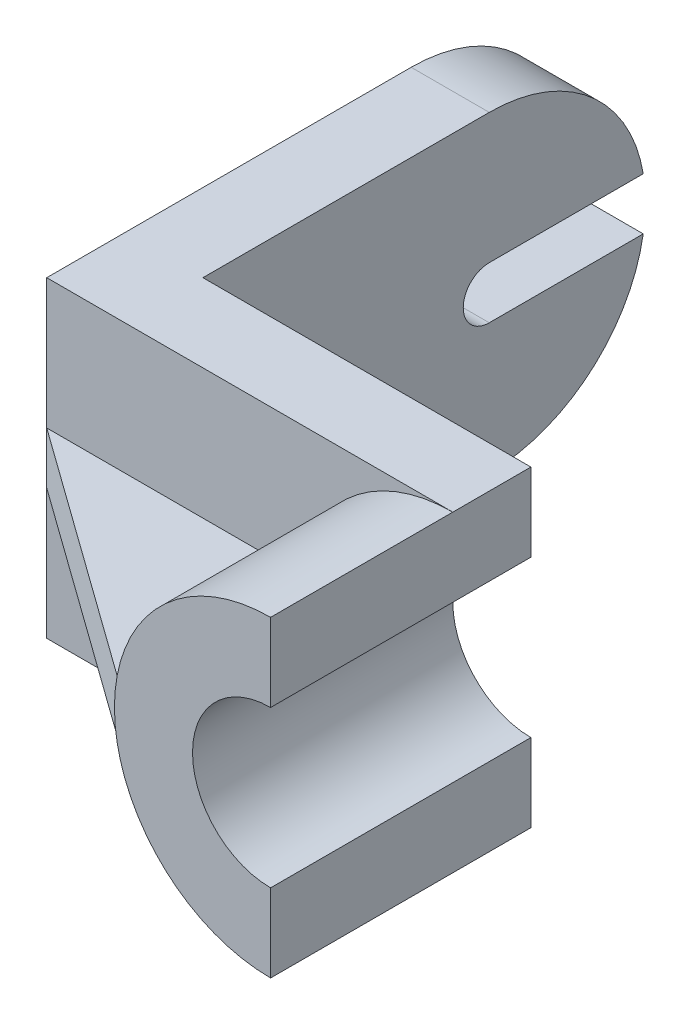
ISO-10303-21;
HEADER;
FILE_DESCRIPTION(('STEP AP214'),'2;1');
FILE_NAME('part.step','',(''),(''),'','','');
FILE_SCHEMA(('AUTOMOTIVE_DESIGN { 1 0 10303 214 1 1 1 1 }'));
ENDSEC;
DATA;
#1=APPLICATION_CONTEXT('core data for automotive mechanical design processes');
#2=APPLICATION_PROTOCOL_DEFINITION('international standard','automotive_design',2000,#1);
#3=PRODUCT_CONTEXT('',#1,'mechanical');
#4=PRODUCT('Part','Part','',(#3));
#5=PRODUCT_RELATED_PRODUCT_CATEGORY('part','',(#4));
#6=PRODUCT_DEFINITION_FORMATION('','',#4);
#7=PRODUCT_DEFINITION_CONTEXT('part definition',#1,'design');
#8=PRODUCT_DEFINITION('design','',#6,#7);
#9=PRODUCT_DEFINITION_SHAPE('','',#8);
#10=(LENGTH_UNIT() NAMED_UNIT(*) SI_UNIT(.MILLI.,.METRE.));
#11=(NAMED_UNIT(*) PLANE_ANGLE_UNIT() SI_UNIT($,.RADIAN.));
#12=(NAMED_UNIT(*) SI_UNIT($,.STERADIAN.) SOLID_ANGLE_UNIT());
#13=UNCERTAINTY_MEASURE_WITH_UNIT(LENGTH_MEASURE(1.E-05),#10,'distance_accuracy_value','');
#14=(GEOMETRIC_REPRESENTATION_CONTEXT(3) GLOBAL_UNCERTAINTY_ASSIGNED_CONTEXT((#13)) GLOBAL_UNIT_ASSIGNED_CONTEXT((#10,
#11,#12)) REPRESENTATION_CONTEXT('',''));
#15=CARTESIAN_POINT('',(0.,0.,0.));
#16=DIRECTION('',(0.,0.,1.));
#17=DIRECTION('',(1.,0.,0.));
#18=AXIS2_PLACEMENT_3D('',#15,#16,#17);
#19=CARTESIAN_POINT('',(15.,-60.,0.));
#20=DIRECTION('',(0.,0.,-1.));
#21=DIRECTION('',(-1.,0.,0.));
#22=AXIS2_PLACEMENT_3D('',#19,#20,#21);
#23=PLANE('',#22);
#24=DIRECTION('',(-1.,0.,0.));
#25=VECTOR('',#24,1.);
#26=CARTESIAN_POINT('',(15.,-25.,0.));
#27=LINE('',#26,#25);
#28=CARTESIAN_POINT('',(48.4196010845019,-25.,0.));
#29=VERTEX_POINT('',#28);
#30=CARTESIAN_POINT('',(0.,-25.,0.));
#31=VERTEX_POINT('',#30);
#32=EDGE_CURVE('E148',#29,#31,#27,.T.);
#33=ORIENTED_EDGE('',*,*,#32,.F.);
#34=CARTESIAN_POINT('',(78.,-30.,0.));
#35=DIRECTION('',(0.,0.,1.));
#36=DIRECTION('',(1.,0.,0.));
#37=AXIS2_PLACEMENT_3D('',#34,#35,#36);
#38=CIRCLE('',#37,30.);
#39=CARTESIAN_POINT('',(78.,0.,0.));
#40=VERTEX_POINT('',#39);
#41=EDGE_CURVE('E246',#40,#29,#38,.T.);
#42=ORIENTED_EDGE('',*,*,#41,.F.);
#43=DIRECTION('',(-1.,0.,0.));
#44=VECTOR('',#43,1.);
#45=CARTESIAN_POINT('',(15.,0.,0.));
#46=LINE('',#45,#44);
#47=CARTESIAN_POINT('',(0.,0.,0.));
#48=VERTEX_POINT('',#47);
#49=EDGE_CURVE('E179',#40,#48,#46,.T.);
#50=ORIENTED_EDGE('',*,*,#49,.T.);
#51=DIRECTION('',(0.,-1.,0.));
#52=VECTOR('',#51,1.);
#53=CARTESIAN_POINT('',(0.,-60.,0.));
#54=LINE('',#53,#52);
#55=EDGE_CURVE('E173',#48,#31,#54,.T.);
#56=ORIENTED_EDGE('',*,*,#55,.T.);
#57=EDGE_LOOP('',(#33,#42,#50,#56));
#58=FACE_BOUND('',#57,.T.);
#59=ADVANCED_FACE('F39',(#58),#23,.F.);
#60=CARTESIAN_POINT('',(15.,-30.,-70.));
#61=DIRECTION('',(-1.,0.,0.));
#62=DIRECTION('',(0.,0.,1.));
#63=AXIS2_PLACEMENT_3D('',#60,#61,#62);
#64=CYLINDRICAL_SURFACE('',#63,30.);
#65=DIRECTION('',(1.,0.,0.));
#66=VECTOR('',#65,1.);
#67=CARTESIAN_POINT('',(0.,-25.,-99.5803989154981));
#68=LINE('',#67,#66);
#69=CARTESIAN_POINT('',(0.,-25.,-99.5803989154981));
#70=VERTEX_POINT('',#69);
#71=CARTESIAN_POINT('',(15.,-25.,-99.5803989154981));
#72=VERTEX_POINT('',#71);
#73=EDGE_CURVE('E219',#70,#72,#68,.T.);
#74=ORIENTED_EDGE('',*,*,#73,.F.);
#75=CARTESIAN_POINT('',(0.,-30.,-70.));
#76=DIRECTION('',(-1.,0.,0.));
#77=DIRECTION('',(0.,0.,1.));
#78=AXIS2_PLACEMENT_3D('',#75,#76,#77);
#79=CIRCLE('',#78,30.);
#80=CARTESIAN_POINT('',(0.,0.,-70.));
#81=VERTEX_POINT('',#80);
#82=EDGE_CURVE('E216',#81,#70,#79,.T.);
#83=ORIENTED_EDGE('',*,*,#82,.F.);
#84=DIRECTION('',(-1.,0.,0.));
#85=VECTOR('',#84,1.);
#86=CARTESIAN_POINT('',(15.,0.,-70.));
#87=LINE('',#86,#85);
#88=CARTESIAN_POINT('',(15.,0.,-70.));
#89=VERTEX_POINT('',#88);
#90=EDGE_CURVE('E194',#89,#81,#87,.T.);
#91=ORIENTED_EDGE('',*,*,#90,.F.);
#92=CARTESIAN_POINT('',(15.,-30.,-70.));
#93=DIRECTION('',(-1.,0.,0.));
#94=DIRECTION('',(0.,0.,1.));
#95=AXIS2_PLACEMENT_3D('',#92,#93,#94);
#96=CIRCLE('',#95,30.);
#97=EDGE_CURVE('E184',#89,#72,#96,.T.);
#98=ORIENTED_EDGE('',*,*,#97,.T.);
#99=EDGE_LOOP('',(#74,#83,#91,#98));
#100=FACE_BOUND('',#99,.T.);
#101=ADVANCED_FACE('F273',(#100),#64,.T.);
#102=CARTESIAN_POINT('',(48.4196010845019,-35.,0.));
#103=VERTEX_POINT('',#102);
#104=CARTESIAN_POINT('',(77.9999999999997,-60.,0.));
#105=VERTEX_POINT('',#104);
#106=EDGE_CURVE('E305',#103,#105,#38,.T.);
#107=ORIENTED_EDGE('',*,*,#106,.F.);
#108=DIRECTION('',(-1.,0.,0.));
#109=VECTOR('',#108,1.);
#110=CARTESIAN_POINT('',(15.,-35.,0.));
#111=LINE('',#110,#109);
#112=CARTESIAN_POINT('',(0.,-35.,0.));
#113=VERTEX_POINT('',#112);
#114=EDGE_CURVE('E303',#103,#113,#111,.T.);
#115=ORIENTED_EDGE('',*,*,#114,.T.);
#116=CARTESIAN_POINT('',(0.,-60.,0.));
#117=VERTEX_POINT('',#116);
#118=EDGE_CURVE('E174',#113,#117,#54,.T.);
#119=ORIENTED_EDGE('',*,*,#118,.T.);
#120=DIRECTION('',(-1.,0.,0.));
#121=VECTOR('',#120,1.);
#122=CARTESIAN_POINT('',(15.,-60.,0.));
#123=LINE('',#122,#121);
#124=EDGE_CURVE('E11',#105,#117,#123,.T.);
#125=ORIENTED_EDGE('',*,*,#124,.F.);
#126=EDGE_LOOP('',(#107,#115,#119,#125));
#127=FACE_BOUND('',#126,.T.);
#128=ADVANCED_FACE('F41',(#127),#23,.F.);
#129=CARTESIAN_POINT('',(15.,-60.,-70.));
#130=DIRECTION('',(0.,1.,0.));
#131=DIRECTION('',(0.,0.,1.));
#132=AXIS2_PLACEMENT_3D('',#129,#130,#131);
#133=PLANE('',#132);
#134=DIRECTION('',(0.,0.,-1.));
#135=VECTOR('',#134,1.);
#136=CARTESIAN_POINT('',(15.,-60.,-70.));
#137=LINE('',#136,#135);
#138=CARTESIAN_POINT('',(15.,-60.,-15.));
#139=VERTEX_POINT('',#138);
#140=CARTESIAN_POINT('',(15.,-60.,-70.));
#141=VERTEX_POINT('',#140);
#142=EDGE_CURVE('E192',#139,#141,#137,.T.);
#143=ORIENTED_EDGE('',*,*,#142,.F.);
#144=DIRECTION('',(1.,0.,0.));
#145=VECTOR('',#144,1.);
#146=CARTESIAN_POINT('',(78.,-60.,-15.));
#147=LINE('',#146,#145);
#148=CARTESIAN_POINT('',(78.,-60.,-15.));
#149=VERTEX_POINT('',#148);
#150=EDGE_CURVE('E240',#139,#149,#147,.T.);
#151=ORIENTED_EDGE('',*,*,#150,.T.);
#152=DIRECTION('',(0.,0.,1.));
#153=VECTOR('',#152,1.);
#154=CARTESIAN_POINT('',(78.,-60.,-15.));
#155=LINE('',#154,#153);
#156=EDGE_CURVE('E243',#149,#105,#155,.T.);
#157=ORIENTED_EDGE('',*,*,#156,.T.);
#158=ORIENTED_EDGE('',*,*,#124,.T.);
#159=DIRECTION('',(0.,0.,-1.));
#160=VECTOR('',#159,1.);
#161=CARTESIAN_POINT('',(0.,-60.,-70.));
#162=LINE('',#161,#160);
#163=CARTESIAN_POINT('',(0.,-60.,-70.));
#164=VERTEX_POINT('',#163);
#165=EDGE_CURVE('E181',#117,#164,#162,.T.);
#166=ORIENTED_EDGE('',*,*,#165,.T.);
#167=DIRECTION('',(-1.,0.,0.));
#168=VECTOR('',#167,1.);
#169=CARTESIAN_POINT('',(15.,-60.,-70.));
#170=LINE('',#169,#168);
#171=EDGE_CURVE('E50',#141,#164,#170,.T.);
#172=ORIENTED_EDGE('',*,*,#171,.F.);
#173=EDGE_LOOP('',(#143,#151,#157,#158,#166,#172));
#174=FACE_BOUND('',#173,.T.);
#175=ADVANCED_FACE('F210',(#174),#133,.F.);
#176=CARTESIAN_POINT('',(15.,0.,0.));
#177=DIRECTION('',(0.,-1.,0.));
#178=DIRECTION('',(0.,0.,-1.));
#179=AXIS2_PLACEMENT_3D('',#176,#177,#178);
#180=PLANE('',#179);
#181=DIRECTION('',(0.,0.,1.));
#182=VECTOR('',#181,1.);
#183=CARTESIAN_POINT('',(0.,0.,0.));
#184=LINE('',#183,#182);
#185=EDGE_CURVE('E182',#81,#48,#184,.T.);
#186=ORIENTED_EDGE('',*,*,#185,.T.);
#187=ORIENTED_EDGE('',*,*,#49,.F.);
#188=DIRECTION('',(0.,0.,1.));
#189=VECTOR('',#188,1.);
#190=CARTESIAN_POINT('',(78.,0.,-15.));
#191=LINE('',#190,#189);
#192=CARTESIAN_POINT('',(78.,0.,-15.));
#193=VERTEX_POINT('',#192);
#194=EDGE_CURVE('E237',#193,#40,#191,.T.);
#195=ORIENTED_EDGE('',*,*,#194,.F.);
#196=DIRECTION('',(-1.,0.,0.));
#197=VECTOR('',#196,1.);
#198=CARTESIAN_POINT('',(0.,0.,-15.));
#199=LINE('',#198,#197);
#200=CARTESIAN_POINT('',(15.,0.,-15.));
#201=VERTEX_POINT('',#200);
#202=EDGE_CURVE('E236',#193,#201,#199,.T.);
#203=ORIENTED_EDGE('',*,*,#202,.T.);
#204=DIRECTION('',(0.,0.,1.));
#205=VECTOR('',#204,1.);
#206=CARTESIAN_POINT('',(15.,0.,0.));
#207=LINE('',#206,#205);
#208=EDGE_CURVE('E190',#89,#201,#207,.T.);
#209=ORIENTED_EDGE('',*,*,#208,.F.);
#210=ORIENTED_EDGE('',*,*,#90,.T.);
#211=EDGE_LOOP('',(#186,#187,#195,#203,#209,#210));
#212=FACE_BOUND('',#211,.T.);
#213=ADVANCED_FACE('F245',(#212),#180,.F.);
#214=CARTESIAN_POINT('',(15.,0.,0.));
#215=DIRECTION('',(-1.,0.,0.));
#216=DIRECTION('',(0.,0.,1.));
#217=AXIS2_PLACEMENT_3D('',#214,#215,#216);
#218=PLANE('',#217);
#219=DIRECTION('',(0.,0.,-1.));
#220=VECTOR('',#219,1.);
#221=CARTESIAN_POINT('',(15.,-35.,-70.));
#222=LINE('',#221,#220);
#223=CARTESIAN_POINT('',(15.,-35.,-70.));
#224=VERTEX_POINT('',#223);
#225=CARTESIAN_POINT('',(15.,-35.,-99.5803989154981));
#226=VERTEX_POINT('',#225);
#227=EDGE_CURVE('E261',#224,#226,#222,.T.);
#228=ORIENTED_EDGE('',*,*,#227,.F.);
#229=CARTESIAN_POINT('',(15.,-30.,-70.));
#230=DIRECTION('',(1.,0.,0.));
#231=DIRECTION('',(0.,0.,-1.));
#232=AXIS2_PLACEMENT_3D('',#229,#230,#231);
#233=CIRCLE('',#232,5.);
#234=CARTESIAN_POINT('',(15.,-25.,-70.));
#235=VERTEX_POINT('',#234);
#236=EDGE_CURVE('E238',#235,#224,#233,.T.);
#237=ORIENTED_EDGE('',*,*,#236,.F.);
#238=DIRECTION('',(0.,0.,1.));
#239=VECTOR('',#238,1.);
#240=CARTESIAN_POINT('',(15.,-25.,-70.));
#241=LINE('',#240,#239);
#242=EDGE_CURVE('E254',#72,#235,#241,.T.);
#243=ORIENTED_EDGE('',*,*,#242,.F.);
#244=ORIENTED_EDGE('',*,*,#97,.F.);
#245=ORIENTED_EDGE('',*,*,#208,.T.);
#246=DIRECTION('',(0.,-1.,0.));
#247=VECTOR('',#246,1.);
#248=CARTESIAN_POINT('',(15.,0.,-15.));
#249=LINE('',#248,#247);
#250=EDGE_CURVE('E65',#201,#139,#249,.T.);
#251=ORIENTED_EDGE('',*,*,#250,.T.);
#252=ORIENTED_EDGE('',*,*,#142,.T.);
#253=EDGE_CURVE('E203',#226,#141,#96,.T.);
#254=ORIENTED_EDGE('',*,*,#253,.F.);
#255=EDGE_LOOP('',(#228,#237,#243,#244,#245,#251,#252,#254));
#256=FACE_BOUND('',#255,.T.);
#257=ADVANCED_FACE('F228',(#256),#218,.F.);
#258=CARTESIAN_POINT('',(0.,0.,0.));
#259=DIRECTION('',(-1.,0.,0.));
#260=DIRECTION('',(0.,0.,1.));
#261=AXIS2_PLACEMENT_3D('',#258,#259,#260);
#262=PLANE('',#261);
#263=ORIENTED_EDGE('',*,*,#118,.F.);
#264=DIRECTION('',(0.,-1.,0.));
#265=VECTOR('',#264,1.);
#266=CARTESIAN_POINT('',(0.,0.,0.));
#267=LINE('',#266,#265);
#268=EDGE_CURVE('E165',#113,#31,#267,.F.);
#269=ORIENTED_EDGE('',*,*,#268,.T.);
#270=ORIENTED_EDGE('',*,*,#55,.F.);
#271=ORIENTED_EDGE('',*,*,#185,.F.);
#272=ORIENTED_EDGE('',*,*,#82,.T.);
#273=DIRECTION('',(0.,0.,1.));
#274=VECTOR('',#273,1.);
#275=CARTESIAN_POINT('',(0.,-25.,-70.));
#276=LINE('',#275,#274);
#277=CARTESIAN_POINT('',(0.,-25.,-70.));
#278=VERTEX_POINT('',#277);
#279=EDGE_CURVE('E253',#70,#278,#276,.T.);
#280=ORIENTED_EDGE('',*,*,#279,.T.);
#281=CARTESIAN_POINT('',(0.,-30.,-70.));
#282=DIRECTION('',(1.,0.,0.));
#283=DIRECTION('',(0.,0.,-1.));
#284=AXIS2_PLACEMENT_3D('',#281,#282,#283);
#285=CIRCLE('',#284,5.);
#286=CARTESIAN_POINT('',(0.,-35.,-70.));
#287=VERTEX_POINT('',#286);
#288=EDGE_CURVE('E252',#278,#287,#285,.T.);
#289=ORIENTED_EDGE('',*,*,#288,.T.);
#290=DIRECTION('',(0.,0.,-1.));
#291=VECTOR('',#290,1.);
#292=CARTESIAN_POINT('',(0.,-35.,-70.));
#293=LINE('',#292,#291);
#294=CARTESIAN_POINT('',(0.,-35.,-99.5803989154981));
#295=VERTEX_POINT('',#294);
#296=EDGE_CURVE('E213',#287,#295,#293,.T.);
#297=ORIENTED_EDGE('',*,*,#296,.T.);
#298=EDGE_CURVE('E205',#295,#164,#79,.T.);
#299=ORIENTED_EDGE('',*,*,#298,.T.);
#300=ORIENTED_EDGE('',*,*,#165,.F.);
#301=EDGE_LOOP('',(#263,#269,#270,#271,#272,#280,#289,#297,#299,#300));
#302=FACE_BOUND('',#301,.T.);
#303=ADVANCED_FACE('F175',(#302),#262,.T.);
#304=DIRECTION('',(1.,0.,0.));
#305=VECTOR('',#304,1.);
#306=CARTESIAN_POINT('',(0.,-35.,-99.5803989154981));
#307=LINE('',#306,#305);
#308=EDGE_CURVE('E267',#295,#226,#307,.T.);
#309=ORIENTED_EDGE('',*,*,#308,.T.);
#310=ORIENTED_EDGE('',*,*,#253,.T.);
#311=ORIENTED_EDGE('',*,*,#171,.T.);
#312=ORIENTED_EDGE('',*,*,#298,.F.);
#313=EDGE_LOOP('',(#309,#310,#311,#312));
#314=FACE_BOUND('',#313,.T.);
#315=ADVANCED_FACE('F202',(#314),#64,.T.);
#316=CARTESIAN_POINT('',(0.,-30.,-70.));
#317=DIRECTION('',(1.,0.,0.));
#318=DIRECTION('',(0.,0.,-1.));
#319=AXIS2_PLACEMENT_3D('',#316,#317,#318);
#320=CYLINDRICAL_SURFACE('',#319,5.);
#321=ORIENTED_EDGE('',*,*,#236,.T.);
#322=DIRECTION('',(1.,0.,0.));
#323=VECTOR('',#322,1.);
#324=CARTESIAN_POINT('',(0.,-35.,-70.));
#325=LINE('',#324,#323);
#326=EDGE_CURVE('E259',#287,#224,#325,.T.);
#327=ORIENTED_EDGE('',*,*,#326,.F.);
#328=ORIENTED_EDGE('',*,*,#288,.F.);
#329=DIRECTION('',(1.,0.,0.));
#330=VECTOR('',#329,1.);
#331=CARTESIAN_POINT('',(0.,-25.,-70.));
#332=LINE('',#331,#330);
#333=EDGE_CURVE('E220',#278,#235,#332,.T.);
#334=ORIENTED_EDGE('',*,*,#333,.T.);
#335=EDGE_LOOP('',(#321,#327,#328,#334));
#336=FACE_BOUND('',#335,.T.);
#337=ADVANCED_FACE('F275',(#336),#320,.F.);
#338=CARTESIAN_POINT('',(0.,-25.,-70.));
#339=DIRECTION('',(0.,1.,0.));
#340=DIRECTION('',(0.,0.,1.));
#341=AXIS2_PLACEMENT_3D('',#338,#339,#340);
#342=PLANE('',#341);
#343=ORIENTED_EDGE('',*,*,#242,.T.);
#344=ORIENTED_EDGE('',*,*,#333,.F.);
#345=ORIENTED_EDGE('',*,*,#279,.F.);
#346=ORIENTED_EDGE('',*,*,#73,.T.);
#347=EDGE_LOOP('',(#343,#344,#345,#346));
#348=FACE_BOUND('',#347,.T.);
#349=ADVANCED_FACE('F279',(#348),#342,.F.);
#350=CARTESIAN_POINT('',(0.,-35.,-70.));
#351=DIRECTION('',(0.,-1.,0.));
#352=DIRECTION('',(0.,0.,-1.));
#353=AXIS2_PLACEMENT_3D('',#350,#351,#352);
#354=PLANE('',#353);
#355=ORIENTED_EDGE('',*,*,#227,.T.);
#356=ORIENTED_EDGE('',*,*,#308,.F.);
#357=ORIENTED_EDGE('',*,*,#296,.F.);
#358=ORIENTED_EDGE('',*,*,#326,.T.);
#359=EDGE_LOOP('',(#355,#356,#357,#358));
#360=FACE_BOUND('',#359,.T.);
#361=ADVANCED_FACE('F270',(#360),#354,.F.);
#362=CARTESIAN_POINT('',(0.,0.,-15.));
#363=DIRECTION('',(0.,0.,-1.));
#364=DIRECTION('',(-1.,0.,0.));
#365=AXIS2_PLACEMENT_3D('',#362,#363,#364);
#366=PLANE('',#365);
#367=ORIENTED_EDGE('',*,*,#150,.F.);
#368=ORIENTED_EDGE('',*,*,#250,.F.);
#369=ORIENTED_EDGE('',*,*,#202,.F.);
#370=DIRECTION('',(0.,-1.,0.));
#371=VECTOR('',#370,1.);
#372=CARTESIAN_POINT('',(78.,-15.,-15.));
#373=LINE('',#372,#371);
#374=CARTESIAN_POINT('',(78.,-15.,-15.));
#375=VERTEX_POINT('',#374);
#376=EDGE_CURVE('E176',#193,#375,#373,.T.);
#377=ORIENTED_EDGE('',*,*,#376,.T.);
#378=CARTESIAN_POINT('',(77.9999999999997,-30.,-15.));
#379=DIRECTION('',(0.,0.,1.));
#380=DIRECTION('',(-1.,0.,0.));
#381=AXIS2_PLACEMENT_3D('',#378,#379,#380);
#382=CIRCLE('',#381,15.);
#383=CARTESIAN_POINT('',(77.9999999999997,-45.,-15.));
#384=VERTEX_POINT('',#383);
#385=EDGE_CURVE('E325',#375,#384,#382,.T.);
#386=ORIENTED_EDGE('',*,*,#385,.T.);
#387=DIRECTION('',(0.,-1.,0.));
#388=VECTOR('',#387,1.);
#389=CARTESIAN_POINT('',(77.9999999999997,-60.,-15.));
#390=LINE('',#389,#388);
#391=EDGE_CURVE('E316',#384,#149,#390,.T.);
#392=ORIENTED_EDGE('',*,*,#391,.T.);
#393=EDGE_LOOP('',(#367,#368,#369,#377,#386,#392));
#394=FACE_BOUND('',#393,.T.);
#395=ADVANCED_FACE('F234',(#394),#366,.T.);
#396=CARTESIAN_POINT('',(77.9999999999998,-30.,35.));
#397=DIRECTION('',(0.,0.,-1.));
#398=DIRECTION('',(-1.,0.,0.));
#399=AXIS2_PLACEMENT_3D('',#396,#397,#398);
#400=CYLINDRICAL_SURFACE('',#399,30.);
#401=DIRECTION('',(0.,0.,-1.));
#402=VECTOR('',#401,1.);
#403=CARTESIAN_POINT('',(48.4196010845018,-35.,35.));
#404=LINE('',#403,#402);
#405=CARTESIAN_POINT('',(48.4196010845018,-35.,34.7742237705084));
#406=VERTEX_POINT('',#405);
#407=EDGE_CURVE('E333',#103,#406,#404,.F.);
#408=ORIENTED_EDGE('',*,*,#407,.F.);
#409=ORIENTED_EDGE('',*,*,#106,.T.);
#410=DIRECTION('',(0.,0.,-1.));
#411=VECTOR('',#410,1.);
#412=CARTESIAN_POINT('',(77.9999999999997,-60.,35.));
#413=LINE('',#412,#411);
#414=CARTESIAN_POINT('',(77.9999999999997,-60.,35.));
#415=VERTEX_POINT('',#414);
#416=EDGE_CURVE('E310',#415,#105,#413,.T.);
#417=ORIENTED_EDGE('',*,*,#416,.F.);
#418=CARTESIAN_POINT('',(77.9999999999998,-30.,35.));
#419=DIRECTION('',(0.,0.,-1.));
#420=DIRECTION('',(-1.,0.,0.));
#421=AXIS2_PLACEMENT_3D('',#418,#419,#420);
#422=CIRCLE('',#421,30.);
#423=CARTESIAN_POINT('',(78.,0.,35.));
#424=VERTEX_POINT('',#423);
#425=EDGE_CURVE('E322',#415,#424,#422,.T.);
#426=ORIENTED_EDGE('',*,*,#425,.T.);
#427=DIRECTION('',(0.,0.,-1.));
#428=VECTOR('',#427,1.);
#429=CARTESIAN_POINT('',(78.,0.,35.));
#430=LINE('',#429,#428);
#431=EDGE_CURVE('E311',#424,#40,#430,.T.);
#432=ORIENTED_EDGE('',*,*,#431,.T.);
#433=ORIENTED_EDGE('',*,*,#41,.T.);
#434=DIRECTION('',(0.,0.,-1.));
#435=VECTOR('',#434,1.);
#436=CARTESIAN_POINT('',(48.4196010845018,-25.,35.));
#437=LINE('',#436,#435);
#438=CARTESIAN_POINT('',(48.4196010845018,-25.,34.7742237705084));
#439=VERTEX_POINT('',#438);
#440=EDGE_CURVE('E153',#29,#439,#437,.F.);
#441=ORIENTED_EDGE('',*,*,#440,.T.);
#442=CARTESIAN_POINT('',(77.9999999999998,-30.,56.0184180238493));
#443=DIRECTION('',(0.583333333333333,0.,-0.812232862067414));
#444=DIRECTION('',(-0.812232862067414,0.,-0.583333333333333));
#445=AXIS2_PLACEMENT_3D('',#442,#443,#444);
#446=ELLIPSE('',#445,36.9352206750656,30.);
#447=EDGE_CURVE('E170',#406,#439,#446,.T.);
#448=ORIENTED_EDGE('',*,*,#447,.F.);
#449=EDGE_LOOP('',(#408,#409,#417,#426,#432,#433,#441,#448));
#450=FACE_BOUND('',#449,.T.);
#451=ADVANCED_FACE('F338',(#450),#400,.T.);
#452=CARTESIAN_POINT('',(77.9999999999997,-60.,35.));
#453=DIRECTION('',(1.,0.,0.));
#454=DIRECTION('',(0.,0.,-1.));
#455=AXIS2_PLACEMENT_3D('',#452,#453,#454);
#456=PLANE('',#455);
#457=ORIENTED_EDGE('',*,*,#391,.F.);
#458=DIRECTION('',(0.,0.,-1.));
#459=VECTOR('',#458,1.);
#460=CARTESIAN_POINT('',(77.9999999999997,-45.,35.));
#461=LINE('',#460,#459);
#462=CARTESIAN_POINT('',(77.9999999999997,-45.,35.));
#463=VERTEX_POINT('',#462);
#464=EDGE_CURVE('E308',#463,#384,#461,.T.);
#465=ORIENTED_EDGE('',*,*,#464,.F.);
#466=DIRECTION('',(0.,-1.,0.));
#467=VECTOR('',#466,1.);
#468=CARTESIAN_POINT('',(77.9999999999997,-60.,35.));
#469=LINE('',#468,#467);
#470=EDGE_CURVE('E314',#463,#415,#469,.T.);
#471=ORIENTED_EDGE('',*,*,#470,.T.);
#472=ORIENTED_EDGE('',*,*,#416,.T.);
#473=ORIENTED_EDGE('',*,*,#156,.F.);
#474=EDGE_LOOP('',(#457,#465,#471,#472,#473));
#475=FACE_BOUND('',#474,.T.);
#476=ADVANCED_FACE('F353',(#475),#456,.T.);
#477=CARTESIAN_POINT('',(77.9999999999997,-30.,35.));
#478=DIRECTION('',(0.,0.,-1.));
#479=DIRECTION('',(-1.,0.,0.));
#480=AXIS2_PLACEMENT_3D('',#477,#478,#479);
#481=CYLINDRICAL_SURFACE('',#480,15.);
#482=ORIENTED_EDGE('',*,*,#464,.T.);
#483=ORIENTED_EDGE('',*,*,#385,.F.);
#484=DIRECTION('',(0.,0.,-1.));
#485=VECTOR('',#484,1.);
#486=CARTESIAN_POINT('',(78.,-15.,35.));
#487=LINE('',#486,#485);
#488=CARTESIAN_POINT('',(78.,-15.,35.));
#489=VERTEX_POINT('',#488);
#490=EDGE_CURVE('E313',#489,#375,#487,.T.);
#491=ORIENTED_EDGE('',*,*,#490,.F.);
#492=CARTESIAN_POINT('',(77.9999999999997,-30.,35.));
#493=DIRECTION('',(0.,0.,1.));
#494=DIRECTION('',(-1.,0.,0.));
#495=AXIS2_PLACEMENT_3D('',#492,#493,#494);
#496=CIRCLE('',#495,15.);
#497=EDGE_CURVE('E330',#489,#463,#496,.T.);
#498=ORIENTED_EDGE('',*,*,#497,.T.);
#499=EDGE_LOOP('',(#482,#483,#491,#498));
#500=FACE_BOUND('',#499,.T.);
#501=ADVANCED_FACE('F352',(#500),#481,.F.);
#502=CARTESIAN_POINT('',(78.,-15.,35.));
#503=DIRECTION('',(1.,0.,0.));
#504=DIRECTION('',(0.,1.,0.));
#505=AXIS2_PLACEMENT_3D('',#502,#503,#504);
#506=PLANE('',#505);
#507=ORIENTED_EDGE('',*,*,#376,.F.);
#508=ORIENTED_EDGE('',*,*,#194,.T.);
#509=ORIENTED_EDGE('',*,*,#431,.F.);
#510=DIRECTION('',(0.,-1.,0.));
#511=VECTOR('',#510,1.);
#512=CARTESIAN_POINT('',(78.,-15.,35.));
#513=LINE('',#512,#511);
#514=EDGE_CURVE('E327',#424,#489,#513,.T.);
#515=ORIENTED_EDGE('',*,*,#514,.T.);
#516=ORIENTED_EDGE('',*,*,#490,.T.);
#517=EDGE_LOOP('',(#507,#508,#509,#515,#516));
#518=FACE_BOUND('',#517,.T.);
#519=ADVANCED_FACE('F341',(#518),#506,.T.);
#520=CARTESIAN_POINT('',(77.9999999999998,-30.,35.));
#521=DIRECTION('',(0.,0.,-1.));
#522=DIRECTION('',(-1.,0.,0.));
#523=AXIS2_PLACEMENT_3D('',#520,#521,#522);
#524=PLANE('',#523);
#525=ORIENTED_EDGE('',*,*,#470,.F.);
#526=ORIENTED_EDGE('',*,*,#497,.F.);
#527=ORIENTED_EDGE('',*,*,#514,.F.);
#528=ORIENTED_EDGE('',*,*,#425,.F.);
#529=EDGE_LOOP('',(#525,#526,#527,#528));
#530=FACE_BOUND('',#529,.T.);
#531=ADVANCED_FACE('F348',(#530),#524,.F.);
#532=CARTESIAN_POINT('',(0.,-30.,0.));
#533=DIRECTION('',(0.583333333333333,0.,-0.812232862067414));
#534=DIRECTION('',(0.812232862067414,0.,0.583333333333333));
#535=AXIS2_PLACEMENT_3D('',#532,#533,#534);
#536=PLANE('',#535);
#537=ORIENTED_EDGE('',*,*,#268,.F.);
#538=DIRECTION('',(0.812232862067414,0.,0.583333333333333));
#539=VECTOR('',#538,1.);
#540=CARTESIAN_POINT('',(0.,-35.,0.));
#541=LINE('',#540,#539);
#542=EDGE_CURVE('E160',#113,#406,#541,.T.);
#543=ORIENTED_EDGE('',*,*,#542,.T.);
#544=ORIENTED_EDGE('',*,*,#447,.T.);
#545=DIRECTION('',(0.812232862067414,0.,0.583333333333333));
#546=VECTOR('',#545,1.);
#547=CARTESIAN_POINT('',(0.,-25.,0.));
#548=LINE('',#547,#546);
#549=EDGE_CURVE('E53',#31,#439,#548,.T.);
#550=ORIENTED_EDGE('',*,*,#549,.F.);
#551=EDGE_LOOP('',(#537,#543,#544,#550));
#552=FACE_BOUND('',#551,.T.);
#553=ADVANCED_FACE('F162',(#552),#536,.F.);
#554=CARTESIAN_POINT('',(39.,-35.,-32.290199457749));
#555=DIRECTION('',(0.,-1.,0.));
#556=DIRECTION('',(0.,0.,-1.));
#557=AXIS2_PLACEMENT_3D('',#554,#555,#556);
#558=PLANE('',#557);
#559=ORIENTED_EDGE('',*,*,#114,.F.);
#560=ORIENTED_EDGE('',*,*,#407,.T.);
#561=ORIENTED_EDGE('',*,*,#542,.F.);
#562=EDGE_LOOP('',(#559,#560,#561));
#563=FACE_BOUND('',#562,.T.);
#564=ADVANCED_FACE('F398',(#563),#558,.T.);
#565=CARTESIAN_POINT('',(39.,-25.,-32.290199457749));
#566=DIRECTION('',(0.,-1.,0.));
#567=DIRECTION('',(0.,0.,-1.));
#568=AXIS2_PLACEMENT_3D('',#565,#566,#567);
#569=PLANE('',#568);
#570=ORIENTED_EDGE('',*,*,#440,.F.);
#571=ORIENTED_EDGE('',*,*,#32,.T.);
#572=ORIENTED_EDGE('',*,*,#549,.T.);
#573=EDGE_LOOP('',(#570,#571,#572));
#574=FACE_BOUND('',#573,.T.);
#575=ADVANCED_FACE('F151',(#574),#569,.F.);
#576=CLOSED_SHELL('',(#59,#101,#128,#175,#213,#257,#303,#315,#337,#349,#361,#395,#451,#476,#501,
#519,#531,#553,#564,#575));
#577=MANIFOLD_SOLID_BREP('B2',#576);
#578=ADVANCED_BREP_SHAPE_REPRESENTATION('',(#18,#577),#14);
#579=SHAPE_DEFINITION_REPRESENTATION(#9,#578);
ENDSEC;
END-ISO-10303-21;
